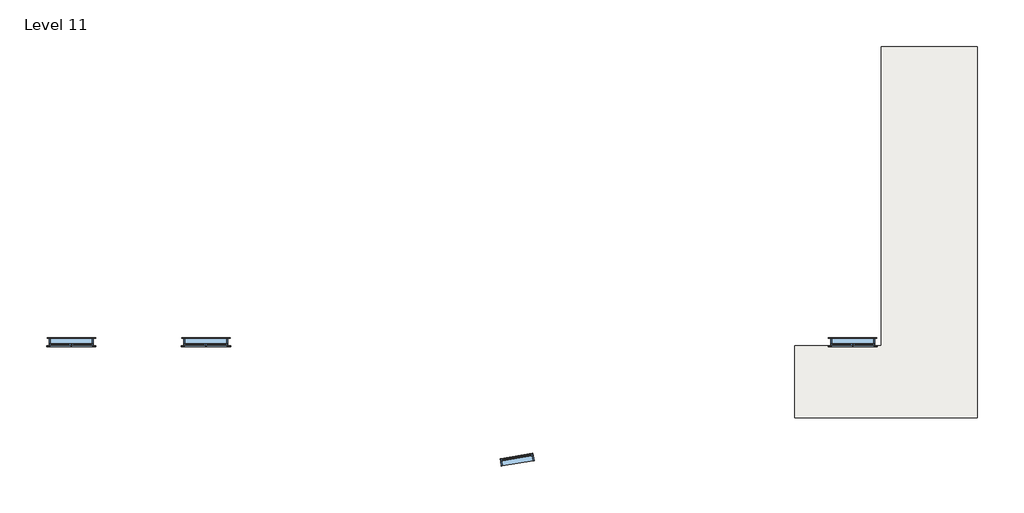
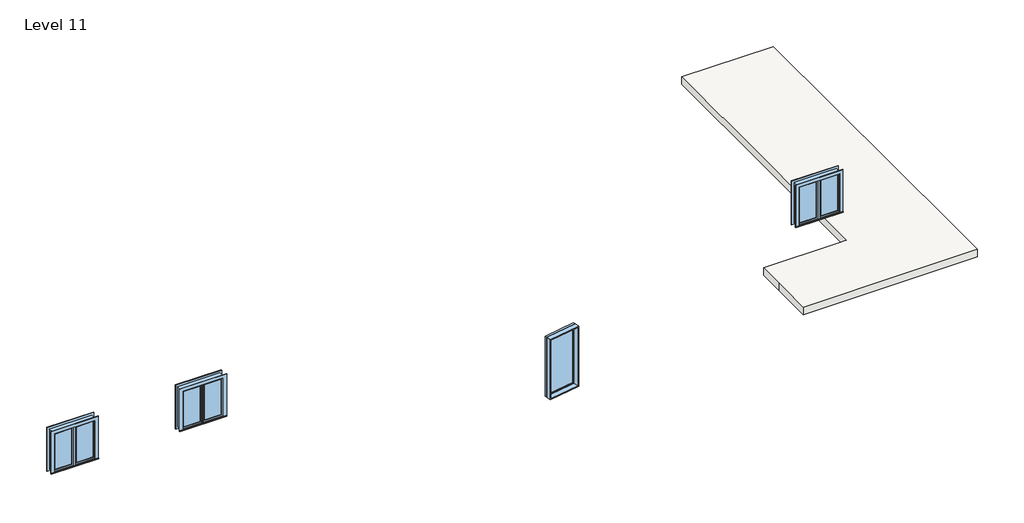
# One storey: 4 windows, 1 slab.
"""IFC4 building model written with IfcOpenShell, lengths in millimetres."""

from ifc_helpers import new_model, si_unit, frame, origin, place, context, project, spatial, polyline, outline, extrude, transform, mapped, element, save
from components import window_0862ab64, window_9a779fa2

model = new_model("IFC4")

# Units and contexts
model_context = context("Model", 3, world=origin())
ifc_project = project(units=[si_unit("LENGTHUNIT", "METRE", prefix="MILLI")], contexts=[model_context])

# Site, building, storey
site = spatial("IfcSite", under=ifc_project)
building = spatial("IfcBuilding", under=site)
storey = spatial("IfcBuildingStorey", under=building, Name="Level 11", Elevation=16383.0)

# Slab
placement = place(None, origin())
element("IfcSlab", 1, ObjectType="9\"", at=placement, inside=storey, context=model_context, shape_type="SweptSolid", body=[
    extrude(outline(polyline([(5058.2494573, -14840.0808221), (5058.2494573, -14078.0808221), (7242.6494573, -14078.0808221), (7445.8494573, -14078.0808221), (7445.8494573, -5848.4808221), (10087.4494573, -5848.4808221), (10087.4494573, -14840.0808221), (10087.4494573, -16059.2808221), (5058.2494573, -16059.2808221), (5058.2494573, -14840.0808221)])), frame((0.0, 0.0, 16154.4), z_axis=(0.0, 0.0, 1.0), x_axis=(1.0, 0.0, 0.0)), (0.0, 0.0, 1.0), 228.6),
])

# Windows
window_shape = window_0862ab64(model_context)
element("IfcWindow", 2, ObjectType="Casement Dbl with Trim : 48\" x 48\"", at=placement, inside=storey, context=model_context, shape_type="MappedRepresentation", body=[
    mapped(window_shape, transform((-11129.6382271, -13957.4308221, 16383.0), x_axis=(-1.0, 0.0, 0.0), y_axis=(0.0, -1.0, 0.0), z_axis=(0.0, 0.0, 1.0))),
])
element("IfcWindow", 3, ObjectType="Casement Dbl with Trim : 48\" x 48\"", at=placement, inside=storey, context=model_context, shape_type="MappedRepresentation", body=[
    mapped(window_shape, transform((-14829.9505427, -13957.4308221, 16383.0), x_axis=(-1.0, 0.0, 0.0), y_axis=(0.0, -1.0, 0.0), z_axis=(0.0, 0.0, 1.0))),
])
element("IfcWindow", 4, ObjectType="Casement Dbl with Trim : 48\" x 48\"", at=placement, inside=storey, context=model_context, shape_type="MappedRepresentation", body=[
    mapped(window_shape, transform((6658.4494573, -13957.4308221, 16383.0), x_axis=(-1.0, 0.0, 0.0), y_axis=(0.0, -1.0, 0.0), z_axis=(0.0, 0.0, 1.0))),
])
window_2_shape = window_9a779fa2(model_context)
element("IfcWindow", 5, ObjectType="Fixed : 36\" x 72\"", at=placement, inside=storey, context=model_context, shape_type="MappedRepresentation", body=[
    mapped(window_2_shape, transform((-2531.9019349, -17202.7478796, 16880.2579834), x_axis=(0.9862985753814015, 0.16497005849734622, 0.0), y_axis=(-0.16497005849734622, 0.9862985753814015, 0.0), z_axis=(0.0, 0.0, 1.0))),
])

save(model, "model.ifc")

# Revit data of these elements
# Type "9\""
#   Assembly Code = "B1010"
#   Function = 0
#   Layers, outside or top first: 0' - 9" no material (function 1)
# Type "Casement Dbl with Trim : 48\" x 48\""
#   Type Mark = "10"
#   Construction Type Id = "GSP4R"
#   Assembly Code = "B2020100"
#   Analytic Construction = "1/8 in Pilkington single glazing"
#   Visual Light Transmittance = 0.9
#   Solar Heat Gain Coefficient = 0.78
#   Heat Transfer Coefficient (U) = 0.6496 BTU/(h·ft²·°F)
#   Height = 4' - 0"
#   Default Sill Height = 3' - 0"
#   Trim Projection - Ext. = 0' - 0 1/2"
#   Trim Projection - Int. = 0' - 0 3/4"
#   Trim Width - Exterior = 0' - 3 1/2"
#   Trim Width - Interior = 0' - 3 1/2"
#   Width = 4' - 0"
#   Window Inset = 0' - 0 3/4"
#   Define Thermal Properties by = 1
#   Glass Pane Material = Glass
#   Sash Material = Sash
#   Trim Exterior Material = Trim
#   Trim Interior Material = Trim
#   Wall Closure = (empty or 0)
# Type "Fixed : 36\" x 72\""
#   Type Mark = "9"
#   Construction Type Id = "GSP4R"
#   Assembly Code = "B2020100"
#   Analytic Construction = "1/8 in Pilkington single glazing"
#   Visual Light Transmittance = 0.9
#   Solar Heat Gain Coefficient = 0.78
#   Heat Transfer Coefficient (U) = 0.6496 BTU/(h·ft²·°F)
#   Height = 6' - 0"
#   Default Sill Height = 1' - 0"
#   Width = 3' - 0"
#   Window Inset = 0' - 0 3/4"
#   Define Thermal Properties by = 1
#   Glass Pane Material = Glass
#   Sash Material = Sash
#   Wall Closure = (empty or 0)
# Element 1 (IfcSlab, "9\"")
#   built-in parameter 1001955 = -1.5708 (stored number, unit not read)
#   Height Offset From Level = 0' - 0"
#   Phase Created = New Construction
#   Materials on its faces: "Default Floor"
# Element 2 (IfcWindow, "Casement Dbl with Trim : 48\" x 48\"")
#   Mark = "37"
#   Phase Created = New Construction
#   Materials on its faces: "Sash", "Trim", "Glass"
# Element 3 (IfcWindow, "Casement Dbl with Trim : 48\" x 48\"")
#   Mark = "38"
#   Phase Created = New Construction
#   Materials on its faces: "Sash", "Trim", "Glass"
# Element 4 (IfcWindow, "Casement Dbl with Trim : 48\" x 48\"")
#   Mark = "56"
#   Phase Created = New Construction
#   Materials on its faces: "Sash", "Trim", "Glass"
# Element 5 (IfcWindow, "Fixed : 36\" x 72\"")
#   Mark = "11"
#   Phase Created = New Construction
#   Materials on its faces: "Sash", "Glass"
# Materials
#   "Glass": class "Glass", colour RGB 0 128 192, transparency 0.75, Description = "Soda Lime Glass", Cost = 0
#   "Sash": class "Wood", colour RGB 224 178 126, transparency 0
#   "Trim": class "Wood", colour RGB 224 178 126, transparency 0
#   "Default Floor": colour RGB 128 128 128, transparency 0
